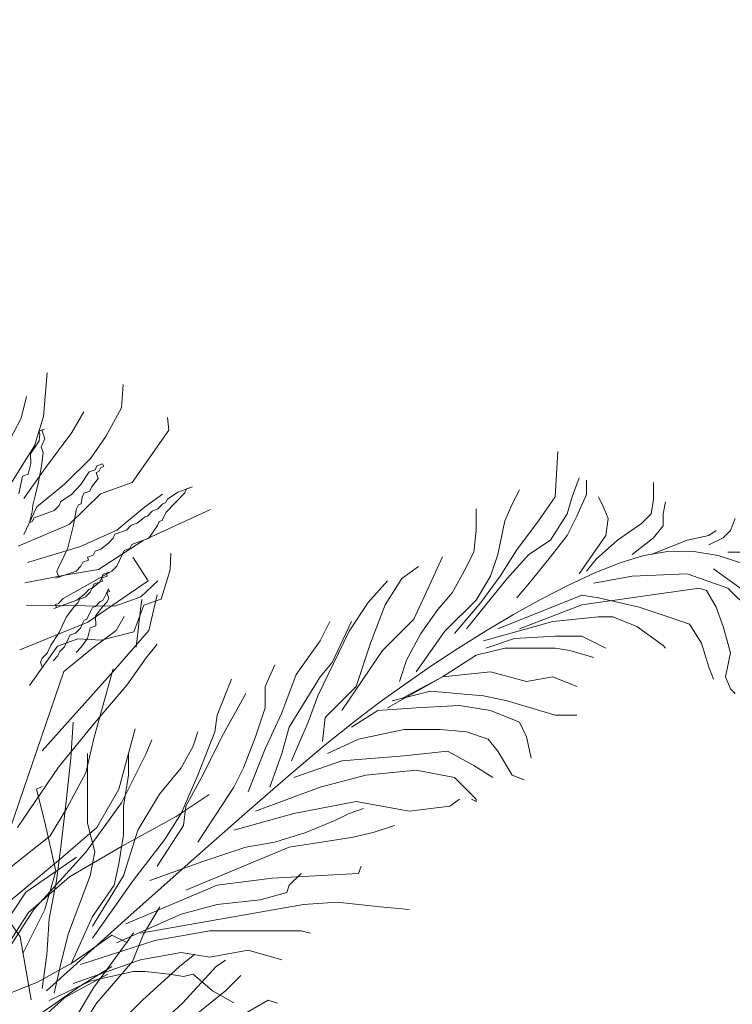
# Model space of a CAD drawing. Units: millimetres. Extents: x 595116 to 630915, y 909473 to 920225.
# Tile 26 of 134: x 629606.562 to 629613.214, y 919171.576 to 919180.767. Entities that reach past the tile are written whole.
import ezdxf

# ---------------------------------------------------------------- set-up
doc = ezdxf.new("R2010")
doc.units = ezdxf.units.MM
doc.layers.add('Dimension', color=3, linetype='Continuous', lineweight=18)
doc.layers.add('L-PLNT', color=85, linetype='Continuous', lineweight=13)
doc.styles.get("Standard").update_dxf_attribs({"font": 'arial.ttf'})
doc.dimstyles.new('ISO-25', dxfattribs={"dimtxt": 9, "dimasz": 6, "dimexe": 1.25, "dimexo": 0.625, "dimtad": 1, "dimlunit": 4, "dimtxsty": 'Standard', "dimcen": 2.5, "dimadec": 0, "dimazin": 0, "dimtfac": 1, "dimtmove": 0, "dimatfit": 3, "dimfxl": 1, "dimarcsym": 0})

# ---------------------------------------------------------------- blocks, each defined once
blk = doc.blocks.new('A$C4FB75ABC')
for p, q in [((2.8876, 3.7608), (2.897, 3.8696)), ((3.0823, 3.7823), (3.0858, 3.8403)), ((2.8322, 3.7571), (2.8454, 3.8105)), ((2.9584, 3.7215), (2.9885, 3.7729)), ((3.043, 3.7114), (3.0823, 3.7823)), ((2.7745, 3.6472), (2.8322, 3.7571)), ((2.8652, 3.6879), (2.8876, 3.7608)), ((3.1994, 3.7272), (3.1962, 3.7584)), ((2.8907, 3.7295), (2.8764, 3.7244)), ((2.8764, 3.7244), (2.8789, 3.7172)), ((2.8835, 3.727), (2.8907, 3.7295)), ((2.8913, 3.7054), (2.8835, 3.727)), ((3.1085, 3.5972), (3.1994, 3.7272)), ((2.8769, 3.7003), (2.856, 3.6684)), ((2.8789, 3.7172), (2.8769, 3.7003)), ((2.8821, 3.6859), (2.8913, 3.7054)), ((2.893, 3.6331), (2.9584, 3.7215)), ((3.0058, 3.6575), (3.043, 3.7114)), ((2.7932, 3.5729), (2.8652, 3.6879)), ((2.8873, 3.6716), (2.8821, 3.6859)), ((4.1608, 3.5609), (4.1668, 3.6742)), ((2.856, 3.6684), (2.8566, 3.6443)), ((2.8833, 3.6377), (2.8873, 3.6716)), ((2.9398, 3.5932), (3.0058, 3.6575)), ((2.8394, 3.5571), (2.893, 3.6331)), ((2.8566, 3.6443), (2.85, 3.6176)), ((2.8746, 3.5941), (2.8833, 3.6377)), ((3.0161, 3.6288), (3.0017, 3.6236)), ((3.0207, 3.6385), (3.0161, 3.6288)), ((3.0187, 3.6216), (3.0258, 3.6242)), ((3.035, 3.6437), (3.0207, 3.6385)), ((3.0258, 3.6242), (3.0304, 3.6339)), ((3.0304, 3.6339), (3.0376, 3.6365)), ((3.0376, 3.6365), (3.035, 3.6437)), ((2.8356, 3.6125), (2.827, 3.5688)), ((2.85, 3.6176), (2.8356, 3.6125)), ((3.0017, 3.6236), (2.9808, 3.5918)), ((3.0075, 3.5852), (3.0238, 3.6072)), ((3.0238, 3.6072), (3.0187, 3.6216)), ((4.2026, 3.5609), (4.2205, 3.6086)), ((4.2384, 3.5668), (4.2384, 3.6026)), ((2.868, 3.5674), (2.8746, 3.5941)), ((2.8712, 3.5361), (2.9398, 3.5932)), ((2.969, 3.5794), (2.9573, 3.5671)), ((2.9808, 3.5918), (2.969, 3.5794)), ((2.9885, 3.5702), (3.0029, 3.5754)), ((3.0029, 3.5754), (3.0075, 3.5852)), ((3.0296, 3.5688), (3.1085, 3.5972)), ((3.2582, 3.5862), (3.2224, 3.5733)), ((3.2393, 3.5713), (3.2439, 3.5811)), ((3.2439, 3.5811), (3.2582, 3.5862)), ((4.0535, 3.543), (4.0714, 3.5788)), ((4.4054, 3.5549), (4.4054, 3.5967)), ((2.8614, 3.5407), (2.868, 3.5674)), ((2.9573, 3.5671), (2.9312, 3.5496)), ((2.9518, 3.4922), (3.0296, 3.5688)), ((2.9819, 3.5435), (2.984, 3.5605)), ((2.984, 3.5605), (2.9885, 3.5702)), ((3.1389, 3.5352), (3.1839, 3.5676)), ((3.1962, 3.5558), (3.1917, 3.5461)), ((3.2224, 3.5733), (3.1962, 3.5558)), ((3.2158, 3.5466), (3.2393, 3.5713)), ((4.1191, 3.5013), (4.1608, 3.5609)), ((4.1907, 3.5192), (4.2026, 3.5609)), ((4.2145, 3.5132), (4.2384, 3.5668)), ((4.2801, 3.537), (4.2682, 3.5609)), ((4.3994, 3.5192), (4.4054, 3.5549)), ((2.8391, 3.4678), (2.8712, 3.5361)), ((2.8594, 3.5238), (2.8614, 3.5407)), ((2.9148, 3.5275), (2.8646, 3.5094)), ((2.9266, 3.5398), (2.9148, 3.5275)), ((2.9312, 3.5496), (2.9266, 3.5398)), ((2.9616, 3.4876), (2.9702, 3.5312)), ((2.9702, 3.5312), (2.9748, 3.541)), ((2.9748, 3.541), (2.9819, 3.5435)), ((3.0703, 3.4781), (3.1389, 3.5352)), ((3.136, 3.4531), (3.303, 3.5294)), ((3.1727, 3.5311), (3.1584, 3.526)), ((3.1845, 3.5435), (3.1727, 3.5311)), ((3.1917, 3.5461), (3.1845, 3.5435)), ((3.1922, 3.522), (3.2158, 3.5466)), ((3.964, 3.4774), (3.964, 3.5311)), ((4.0356, 3.5013), (4.0535, 3.543)), ((4.2921, 3.5072), (4.2801, 3.537)), ((4.4293, 3.5192), (4.4352, 3.549)), ((2.8528, 3.4971), (2.8594, 3.5238)), ((2.8646, 3.5094), (2.86, 3.4997)), ((3.1394, 3.5111), (3.1205, 3.4961)), ((3.1466, 3.5136), (3.1394, 3.5111)), ((3.1584, 3.526), (3.1466, 3.5136)), ((3.1759, 3.4999), (3.1831, 3.5024)), ((3.1831, 3.5024), (3.1922, 3.522)), ((4.1489, 3.4536), (4.1907, 3.5192)), ((4.1907, 3.4655), (4.2145, 3.5132)), ((4.2861, 3.4655), (4.2921, 3.5072)), ((4.3756, 3.4953), (4.3994, 3.5192)), ((4.4293, 3.4893), (4.4293, 3.5192)), ((4.5963, 3.4774), (4.6082, 3.5072)), ((2.8253, 3.4385), (2.9518, 3.4922)), ((2.86, 3.4997), (2.8528, 3.4971)), ((2.9484, 3.4342), (2.9616, 3.4876)), ((2.9797, 3.4374), (3.0703, 3.4781)), ((3.0944, 3.4786), (3.0657, 3.4683)), ((3.1062, 3.491), (3.0944, 3.4786)), ((3.1205, 3.4961), (3.1062, 3.491)), ((3.1503, 3.4583), (3.1713, 3.4901)), ((3.1713, 3.4901), (3.1759, 3.4999)), ((3.958, 3.4238), (3.964, 3.4774)), ((4.0177, 3.4178), (4.0356, 3.5013)), ((4.0654, 3.4297), (4.1191, 3.5013)), ((4.3159, 3.4536), (4.3756, 3.4953)), ((4.4054, 3.4595), (4.4293, 3.4893)), ((4.5426, 3.4655), (4.5605, 3.4774)), ((4.5784, 3.4595), (4.5963, 3.4774)), ((3.0244, 3.3805), (3.136, 3.4531)), ((3.0611, 3.4586), (3.0494, 3.4462)), ((3.0657, 3.4683), (3.0611, 3.4586)), ((3.1073, 3.4428), (3.1503, 3.4583)), ((4.0952, 3.4178), (4.1489, 3.4536)), ((4.1489, 3.4118), (4.1907, 3.4655)), ((4.2205, 3.3701), (4.2861, 3.4655)), ((4.2622, 3.4059), (4.3159, 3.4536)), ((4.3517, 3.4178), (4.4054, 3.4595)), ((4.3994, 3.4178), (4.4889, 3.4536)), ((4.4889, 3.4536), (4.5426, 3.4655)), ((4.5426, 3.4416), (4.5784, 3.4595)), ((2.848, 3.3981), (2.9797, 3.4374)), ((2.9392, 3.4147), (2.9484, 3.4342)), ((3.0304, 3.4313), (3.0161, 3.4262)), ((3.0494, 3.4462), (3.0304, 3.4313)), ((3.0884, 3.4279), (3.1027, 3.433)), ((3.1027, 3.433), (3.1073, 3.4428)), ((4.0237, 3.3641), (4.0654, 3.4297)), ((2.9254, 3.3854), (2.9392, 3.4147)), ((2.9997, 3.4041), (2.9854, 3.3989)), ((3.0115, 3.4164), (2.9972, 3.4112)), ((2.9972, 3.4112), (2.9997, 3.4041)), ((3.0161, 3.4262), (3.0115, 3.4164)), ((3.07, 3.3888), (3.0884, 3.4279)), ((3.1481, 3.3521), (3.1105, 3.4115)), ((3.2028, 3.3799), (3.2043, 3.4209)), ((3.8447, 3.3343), (3.8805, 3.4118)), ((3.9342, 3.3761), (3.958, 3.4238)), ((3.9998, 3.3641), (4.0177, 3.4178)), ((4.0415, 3.3582), (4.0952, 3.4178)), ((4.1012, 3.3522), (4.1489, 3.4118)), ((4.2384, 3.3761), (4.2622, 3.4059)), ((4.322, 3.3969), (4.3813, 3.4152)), ((4.3813, 3.4152), (4.4396, 3.4254)), ((4.4396, 3.4254), (4.5001, 3.426)), ((4.5001, 3.426), (4.5657, 3.4153)), ((4.5657, 3.4153), (4.6395, 3.3917)), ((4.5903, 3.4238), (4.6201, 3.4238)), ((2.9208, 3.3757), (2.9254, 3.3854)), ((2.9403, 3.3665), (3.0244, 3.3805)), ((2.9808, 3.3891), (2.969, 3.3768)), ((2.9854, 3.3989), (2.9808, 3.3891)), ((3.0583, 3.3765), (3.07, 3.3888)), ((3.1805, 3.307), (3.2028, 3.3799)), ((3.7791, 3.3582), (3.8208, 3.388)), ((4.2593, 3.3722), (4.322, 3.3969)), ((4.5545, 3.382), (4.6858, 3.2866)), ((2.8419, 3.3473), (2.9403, 3.3665)), ((2.969, 3.3768), (2.9188, 3.3587)), ((2.9188, 3.3587), (2.926, 3.3613)), ((2.926, 3.3613), (2.9208, 3.3757)), ((2.9369, 3.3085), (3.0583, 3.3765)), ((3.0322, 3.359), (3.0276, 3.3492)), ((3.0367, 3.3687), (3.0322, 3.359)), ((3.0322, 3.359), (3.0465, 3.3642)), ((3.0347, 3.3518), (3.0322, 3.359)), ((3.0511, 3.3739), (3.0367, 3.3687)), ((3.0439, 3.3713), (3.0511, 3.3739)), ((3.0465, 3.3642), (3.0439, 3.3713)), ((3.7373, 3.2926), (3.7791, 3.3582)), ((3.9044, 3.3224), (3.9342, 3.3761)), ((3.964, 3.3045), (3.9998, 3.3641)), ((3.9759, 3.2986), (4.0237, 3.3641)), ((3.9879, 3.2926), (4.0415, 3.3582)), ((4.1935, 3.342), (4.2593, 3.3722)), ((4.2563, 3.3463), (4.3517, 3.3641)), ((4.3517, 3.3641), (4.4889, 3.3701)), ((4.4889, 3.3701), (4.5903, 3.3343)), ((3.0015, 3.3317), (2.9897, 3.3194)), ((2.9986, 3.2497), (3.1481, 3.3521)), ((3.0086, 3.3343), (3.0015, 3.3317)), ((3.004, 3.3246), (3.0086, 3.3343)), ((3.0276, 3.3492), (3.0086, 3.3343)), ((3.0086, 3.3343), (3.0132, 3.3441)), ((3.0132, 3.3441), (3.0347, 3.3518)), ((3.0497, 3.3329), (3.0451, 3.3231)), ((3.0522, 3.3257), (3.0497, 3.3329)), ((3.1297, 3.313), (3.1722, 3.3526)), ((3.6956, 3.2986), (3.7433, 3.3522)), ((3.8089, 3.2568), (3.8447, 3.3343)), ((4.0654, 3.3105), (4.1012, 3.3522)), ((4.1256, 3.3072), (4.1935, 3.342)), ((4.2265, 3.2926), (4.5187, 3.3343)), ((4.5187, 3.3343), (4.5366, 3.3284)), ((4.5903, 3.3343), (4.644, 3.2807)), ((2.9251, 3.2962), (2.9369, 3.3085)), ((2.9897, 3.3194), (2.9708, 3.3045)), ((2.9733, 3.2973), (2.9779, 3.3071)), ((2.9779, 3.3071), (2.9923, 3.3122)), ((2.9923, 3.3122), (3.004, 3.3246)), ((3.0359, 3.3036), (3.0405, 3.3134)), ((3.0405, 3.3134), (3.0451, 3.3231)), ((3.0451, 3.3231), (3.0522, 3.3257)), ((3.0451, 3.3231), (3.0502, 3.3088)), ((3.0502, 3.3088), (3.0456, 3.299)), ((3.0651, 3.2898), (3.1297, 3.313)), ((3.1303, 3.2889), (3.1323, 3.3059)), ((3.1374, 3.2915), (3.1805, 3.307)), ((3.1501, 3.2292), (3.1706, 3.3178)), ((3.8686, 3.2807), (3.9044, 3.3224)), ((4.0177, 3.233), (4.2265, 3.3164)), ((4.0565, 3.2687), (4.1256, 3.3072)), ((4.2265, 3.3164), (4.2682, 3.3105)), ((4.2682, 3.3105), (4.3696, 3.2866)), ((4.5366, 3.3284), (4.5605, 3.2866)), ((2.8457, 3.2919), (3.0651, 3.2898)), ((2.9708, 3.3045), (2.9134, 3.2838)), ((2.9134, 3.2838), (2.9206, 3.2864)), ((2.918, 3.2936), (2.9251, 3.2962)), ((2.9206, 3.2864), (2.918, 3.2936)), ((2.9452, 3.2629), (2.9616, 3.285)), ((2.9616, 3.285), (2.9733, 3.2973)), ((3.0052, 3.2763), (3.0098, 3.2861)), ((3.0098, 3.2861), (3.0169, 3.2887)), ((3.0169, 3.2887), (3.0287, 3.301)), ((3.0339, 3.2867), (3.0175, 3.2646)), ((3.0287, 3.301), (3.0359, 3.3036)), ((3.0456, 3.299), (3.0339, 3.2867)), ((3.1125, 3.2258), (3.1374, 3.2915)), ((3.1182, 3.1873), (3.1303, 3.2889)), ((3.6479, 3.227), (3.6956, 3.2986)), ((3.7015, 3.1972), (3.7373, 3.2926)), ((3.8865, 3.227), (3.964, 3.3045)), ((3.9103, 3.2211), (3.9759, 3.2986)), ((3.9401, 3.233), (3.9879, 3.2926)), ((4.0714, 3.233), (4.2265, 3.2926)), ((4.3696, 3.2866), (4.4412, 3.2628)), ((4.5605, 3.2866), (4.5784, 3.2389)), ((2.936, 3.2434), (2.9452, 3.2629)), ((2.996, 3.2568), (3.0052, 3.2763)), ((3.0175, 3.2646), (3.0181, 3.2405)), ((3.0684, 3.2292), (3.0888, 3.2633)), ((3.8268, 3.2211), (3.8686, 3.2807)), ((3.9871, 3.2274), (4.0565, 3.2687)), ((4.1549, 3.2509), (4.2682, 3.2628)), ((4.2682, 3.2628), (4.304, 3.2628)), ((4.304, 3.2628), (4.3637, 3.2389)), ((4.4412, 3.2628), (4.4949, 3.2449)), ((2.829, 3.1805), (2.9986, 3.2497)), ((2.9269, 3.2238), (2.936, 3.2434)), ((2.9679, 3.2224), (2.9797, 3.2347)), ((2.9797, 3.2347), (2.9842, 3.2445)), ((2.9842, 3.2445), (2.9888, 3.2542)), ((2.9888, 3.2542), (2.996, 3.2568)), ((3.0038, 3.2353), (2.9972, 3.2086)), ((3.0181, 3.2405), (3.0038, 3.2353)), ((3.5763, 3.2032), (3.6001, 3.2509)), ((3.6061, 3.1495), (3.6538, 3.2509)), ((3.7314, 3.1793), (3.8089, 3.2568)), ((3.9819, 3.2032), (4.1549, 3.2509)), ((4.3637, 3.2389), (4.4054, 3.2091)), ((4.4949, 3.2449), (4.5247, 3.1972)), ((4.5784, 3.2389), (4.5963, 3.1734)), ((2.9059, 3.192), (2.9269, 3.2238)), ((2.9229, 3.19), (2.9731, 3.208)), ((2.949, 3.2075), (2.9535, 3.2172)), ((2.9535, 3.2172), (2.9679, 3.2224)), ((2.9731, 3.208), (3.031, 3.2046)), ((2.9972, 3.2086), (2.9808, 3.1865)), ((3.0139, 3.1884), (3.0684, 3.2292)), ((3.031, 3.2046), (3.1125, 3.2258)), ((3.0616, 3.1271), (3.1501, 3.2292)), ((3.5703, 3.066), (3.6479, 3.227)), ((3.791, 3.1555), (3.8268, 3.2211)), ((3.8149, 3.1257), (3.8865, 3.227)), ((3.9185, 3.1843), (3.9871, 3.2274)), ((3.9879, 3.1853), (4.0594, 3.2091)), ((4.0594, 3.2091), (4.1608, 3.2151)), ((4.1608, 3.2151), (4.2265, 3.2151)), ((4.2265, 3.2151), (4.2861, 3.1853)), ((4.4054, 3.2091), (4.4293, 3.1912)), ((2.8529, 3.0918), (2.9229, 3.19)), ((2.8967, 3.1725), (2.9059, 3.192)), ((2.928, 3.1756), (2.9398, 3.188)), ((2.9389, 3.1271), (3.0139, 3.1884)), ((2.9398, 3.188), (2.949, 3.2075)), ((2.9808, 3.1865), (2.969, 3.1742)), ((3.1433, 3.1611), (3.1706, 3.1952)), ((3.5166, 3.1197), (3.5763, 3.2032)), ((3.6658, 3.0899), (3.7015, 3.1972)), ((3.8516, 3.1401), (3.9185, 3.1843)), ((3.964, 3.1674), (4.0356, 3.1853)), ((4.0356, 3.1853), (4.1072, 3.1853)), ((4.1072, 3.1853), (4.1608, 3.1853)), ((4.1608, 3.1853), (4.1966, 3.1793)), ((4.4293, 3.1912), (4.4352, 3.1853)), ((4.5247, 3.1972), (4.5426, 3.1376)), ((2.8804, 3.1504), (2.885, 3.1601)), ((2.885, 3.1601), (2.8967, 3.1725)), ((2.9117, 3.1535), (2.9234, 3.1659)), ((2.9234, 3.1659), (2.928, 3.1756)), ((3.0956, 3.093), (3.1433, 3.1611)), ((3.63, 3.0303), (3.7314, 3.1793)), ((3.8805, 3.1137), (3.964, 3.1674)), ((4.1966, 3.1793), (4.2563, 3.1614)), ((4.5963, 3.1734), (4.5844, 3.1137)), ((2.8856, 3.136), (2.8804, 3.1504)), ((3.4391, 3.0899), (3.4629, 3.1436)), ((3.5763, 3.1137), (3.6061, 3.1495)), ((3.7731, 3.1018), (3.791, 3.1555)), ((3.7873, 3.0958), (3.8516, 3.1401)), ((4.5426, 3.1376), (4.5545, 3.1078)), ((2.7823, 2.6709), (2.9389, 3.1271)), ((2.8844, 2.9296), (3.0616, 3.1271)), ((3.0139, 2.9637), (3.0616, 3.1339)), ((3.4808, 3.0243), (3.5166, 3.1197)), ((3.4987, 2.9885), (3.5763, 3.1137)), ((3.7433, 3.0362), (3.8805, 3.1137)), ((3.7791, 3.0601), (3.8805, 3.1137)), ((3.8805, 3.1137), (3.9998, 3.1257)), ((3.9998, 3.1257), (4.0893, 3.1018)), ((4.0893, 3.1018), (4.1549, 3.1137)), ((4.1549, 3.1137), (4.2145, 3.0899)), ((4.5844, 3.1137), (4.5963, 3.0839)), ((3.0139, 2.9977), (3.0956, 3.093)), ((3.3198, 3.0184), (3.3556, 3.1078)), ((3.4391, 3.0362), (3.4391, 3.0899)), ((3.5882, 3.0124), (3.6658, 3.0899)), ((3.7254, 3.0513), (3.7873, 3.0958)), ((3.3317, 2.9647), (3.3914, 3.072)), ((3.5465, 3.0005), (3.5703, 3.066)), ((3.7552, 3.0541), (3.8507, 3.078)), ((3.8507, 3.078), (3.9819, 3.066)), ((3.9819, 3.066), (4.0415, 3.0541)), ((4.5963, 3.0839), (4.6082, 3.072)), ((3.6611, 3.0024), (3.7254, 3.0513)), ((3.8149, 3.0362), (3.9222, 3.0422)), ((3.9222, 3.0422), (3.9998, 3.0303)), ((4.0415, 3.0541), (4.1608, 3.0184)), ((3.3138, 2.9766), (3.3198, 3.0184)), ((3.4152, 2.9647), (3.4391, 3.0362)), ((3.4391, 2.9349), (3.4808, 3.0243)), ((3.5822, 2.9528), (3.5882, 3.0124)), ((3.6538, 2.9885), (3.7194, 3.0303)), ((3.7194, 3.0303), (3.8149, 3.0362)), ((3.9998, 3.0303), (4.0714, 3.0005)), ((4.1608, 3.0184), (4.2145, 3.0184)), ((2.9253, 2.8888), (3.0139, 2.9977)), ((2.9559, 2.911), (2.9619, 3.0005)), ((3.4808, 2.923), (3.4987, 2.9885)), ((3.5047, 2.9051), (3.5465, 3.0005)), ((3.5886, 2.9442), (3.6611, 3.0024)), ((4.0714, 3.0005), (4.0893, 2.9647)), ((2.9935, 2.8751), (3.0139, 2.9637)), ((3.0752, 2.8343), (3.1161, 2.9841)), ((3.2601, 2.9408), (3.2721, 2.9766)), ((3.2721, 2.8693), (3.3138, 2.9766)), ((3.284, 2.8693), (3.3317, 2.9647)), ((3.3854, 2.8872), (3.4152, 2.9647)), ((3.6717, 2.9587), (3.7851, 2.9826)), ((3.7851, 2.9826), (3.8745, 2.9826)), ((3.8745, 2.9826), (3.9401, 2.9766)), ((3.9401, 2.9766), (3.9938, 2.9587)), ((4.0893, 2.9647), (4.1012, 2.911)), ((3.1433, 2.9228), (3.157, 2.9569)), ((3.2303, 2.8872), (3.2601, 2.9408)), ((3.5019, 2.8714), (3.5886, 2.9442)), ((3.5942, 2.923), (3.6717, 2.9587)), ((3.9938, 2.9587), (4.0177, 2.9289)), ((2.9977, 2.8216), (2.9977, 2.923)), ((3.082, 2.8002), (3.1433, 2.9228)), ((3.0991, 2.8693), (3.0991, 2.923)), ((3.3973, 2.8276), (3.4391, 2.9349)), ((3.451, 2.8395), (3.4808, 2.923)), ((3.63, 2.9051), (3.7851, 2.917)), ((3.7851, 2.917), (3.8924, 2.9289)), ((3.8924, 2.9289), (3.958, 2.8932)), ((4.0177, 2.9289), (4.0535, 2.8693)), ((2.944, 2.8037), (2.9559, 2.911)), ((3.5107, 2.8633), (3.63, 2.9051)), ((3.958, 2.8932), (4.0058, 2.8633)), ((2.8231, 2.739), (2.9253, 2.8888)), ((2.9458, 2.7866), (2.9935, 2.8751)), ((3.0872, 2.7918), (3.0991, 2.8693)), ((3.1766, 2.8216), (3.2303, 2.8872)), ((3.2303, 2.7739), (3.2721, 2.8693)), ((3.2422, 2.7918), (3.284, 2.8693)), ((3.3615, 2.8395), (3.3854, 2.8872)), ((3.3951, 2.779), (3.5019, 2.8714)), ((3.5763, 2.8395), (3.6896, 2.8693)), ((3.6896, 2.8693), (3.8149, 2.8812)), ((3.8149, 2.8812), (3.9103, 2.8633)), ((4.0535, 2.8693), (4.0833, 2.8574)), ((2.8708, 2.8343), (2.8844, 2.8411)), ((3.9103, 2.8633), (3.964, 2.8097)), ((2.8913, 2.7526), (2.8708, 2.8343)), ((2.9977, 2.7501), (2.9977, 2.8216)), ((3.0207, 2.739), (3.0752, 2.8343)), ((3.1229, 2.7322), (3.1766, 2.8216)), ((3.2183, 2.7662), (3.3, 2.8207)), ((3.2721, 2.7024), (3.3615, 2.8395)), ((3.4152, 2.7799), (3.5763, 2.8395)), ((2.9321, 2.6964), (2.944, 2.8037)), ((2.9935, 2.6777), (3.082, 2.8002)), ((3.0872, 2.7203), (3.0872, 2.7918)), ((3.2363, 2.7441), (3.2422, 2.7918)), ((3.5107, 2.7739), (3.6658, 2.8037)), ((3.6658, 2.8037), (3.797, 2.7799)), ((3.797, 2.7799), (3.8984, 2.7918)), ((3.8984, 2.7918), (3.9222, 2.8097)), ((3.964, 2.8037), (3.9521, 2.8097)), ((3.964, 2.8097), (3.964, 2.8037)), ((2.9049, 2.7185), (2.9458, 2.7866)), ((3.1886, 2.7083), (3.2303, 2.7739)), ((3.2623, 2.6619), (3.3951, 2.779)), ((3.3615, 2.7322), (3.5107, 2.7739)), ((3.6121, 2.756), (3.6479, 2.7739)), ((3.6479, 2.7739), (3.6837, 2.7858)), ((2.9185, 2.63), (2.8913, 2.7526)), ((3.0156, 2.6785), (2.9977, 2.7501)), ((3.082, 2.6913), (3.2183, 2.7662)), ((3.1707, 2.6428), (3.2363, 2.7441)), ((3.5405, 2.7262), (3.6121, 2.756)), ((3.7075, 2.7262), (3.7612, 2.7441)), ((2.7414, 2.5891), (2.9049, 2.7185)), ((2.9253, 2.6572), (3.0207, 2.739)), ((3.0752, 2.6487), (3.0872, 2.7203)), ((3.0872, 2.6189), (3.1229, 2.7322)), ((3.4629, 2.7024), (3.5405, 2.7262)), ((3.6538, 2.7143), (3.7075, 2.7262)), ((2.9201, 2.607), (2.9321, 2.6964)), ((3.111, 2.607), (3.1886, 2.7083)), ((3.3914, 2.6904), (3.4629, 2.7024)), ((3.4987, 2.6904), (3.6538, 2.7143)), ((2.864, 2.5347), (2.9935, 2.6777)), ((2.9526, 2.6164), (3.082, 2.6913)), ((3.0036, 2.6189), (3.0156, 2.6785)), ((3.2422, 2.5831), (3.4987, 2.6904)), ((3.284, 2.6547), (3.3914, 2.6904)), ((2.7209, 2.487), (2.9253, 2.6572)), ((2.8442, 2.5778), (2.9704, 2.6651)), ((3.0633, 2.5951), (3.0752, 2.6487)), ((3.0976, 2.5149), (3.2623, 2.6619)), ((3.1528, 2.607), (3.284, 2.6547)), ((2.8913, 2.5347), (2.9185, 2.63)), ((3.457, 2.6129), (3.6717, 2.6249)), ((3.4987, 2.5951), (3.5286, 2.6249)), ((3.6717, 2.6249), (3.6777, 2.6428)), ((2.8504, 2.5279), (2.9526, 2.6164)), ((2.9022, 2.5116), (2.9201, 2.607)), ((2.95, 2.4758), (3.0036, 2.6189)), ((3.0096, 2.4937), (3.0872, 2.6189)), ((3.0096, 2.4639), (3.111, 2.607)), ((3.3198, 2.5951), (3.457, 2.6129)), ((2.786, 2.4905), (2.8442, 2.5778)), ((3.0096, 2.5176), (3.0633, 2.5951)), ((3.0931, 2.4997), (3.3198, 2.5951)), ((3.4272, 2.5593), (3.4928, 2.5772)), ((3.4928, 2.5772), (3.4987, 2.5951)), ((2.8299, 2.4666), (2.7686, 2.5551)), ((3.1289, 2.4758), (3.5345, 2.5474)), ((3.2303, 2.5235), (3.3198, 2.5474)), ((3.3198, 2.5474), (3.4272, 2.5593)), ((3.5345, 2.5474), (3.618, 2.5533)), ((3.618, 2.5533), (3.7254, 2.5414)), ((2.7891, 2.4325), (2.8504, 2.5279)), ((2.8027, 2.4393), (2.864, 2.5347)), ((2.8368, 2.4257), (2.8913, 2.5347)), ((3.0693, 2.452), (3.2303, 2.5235)), ((3.1365, 2.4734), (3.1774, 2.5415)), ((3.7254, 2.5414), (3.797, 2.5354)), ((2.895, 2.333), (3.0976, 2.5149)), ((2.8963, 2.4222), (2.9022, 2.5116)), ((2.9559, 2.3983), (3.0096, 2.5176)), ((2.9321, 2.4043), (2.95, 2.4758)), ((3.0962, 2.4544), (3.1115, 2.4773)), ((3.1093, 2.4053), (3.1365, 2.4734)), ((3.1647, 2.4579), (3.3019, 2.4818)), ((3.3019, 2.4818), (3.4152, 2.4818)), ((3.4152, 2.4818), (3.5286, 2.4818)), ((3.5286, 2.4818), (3.5524, 2.4758)), ((2.8572, 2.31), (2.8299, 2.4666)), ((2.9607, 2.4032), (3.0578, 2.4711)), ((2.9798, 2.3983), (3.1647, 2.4579)), ((3.0123, 2.3401), (3.0962, 2.4544)), ((3.0578, 2.4711), (3.0966, 2.4517)), ((3.1289, 2.4102), (3.2303, 2.4281)), ((3.2303, 2.4281), (3.3019, 2.4162)), ((3.3019, 2.4162), (3.3973, 2.4341)), ((3.3973, 2.4341), (3.4808, 2.4102)), ((2.8733, 2.3546), (2.9607, 2.4032)), ((2.8844, 2.3387), (2.8963, 2.4222)), ((2.9142, 2.3268), (2.9321, 2.4043)), ((2.9619, 2.3506), (3.1289, 2.4102)), ((3.0207, 2.3031), (3.1093, 2.4053)), ((3.2259, 2.3934), (3.264, 2.4239)), ((3.3174, 2.3934), (3.3403, 2.4087)), ((2.9801, 2.3449), (3.0578, 2.3935)), ((3.0036, 2.3566), (3.111, 2.3804)), ((3.111, 2.3804), (3.1408, 2.3804)), ((3.1344, 2.3096), (3.2259, 2.3934)), ((3.1408, 2.3804), (3.2005, 2.3745)), ((3.2335, 2.302), (3.3174, 2.3934)), ((2.7277, 2.2964), (2.8733, 2.3546)), ((2.9022, 2.3089), (3.0036, 2.3566)), ((2.9413, 2.3158), (3.0481, 2.3741)), ((3.2005, 2.3745), (3.2363, 2.3685)), ((3.2363, 2.3685), (3.2601, 2.3745)), ((3.2601, 2.3745), (3.3079, 2.3327)), ((3.3403, 2.3324), (3.3784, 2.3706)), ((2.8539, 2.2576), (2.9801, 2.3449)), ((2.9666, 2.2638), (3.0123, 2.3401)), ((3.264, 2.2715), (3.3403, 2.3324)), ((3.3079, 2.3327), (3.3615, 2.3029)), ((2.8539, 2.2382), (2.9413, 2.3158)), ((2.9321, 2.167), (3.0207, 2.3031)), ((3.0505, 2.2257), (3.1344, 2.3096)), ((3.142, 2.2181), (3.2335, 2.302)), ((3.3937, 2.2791), (3.447, 2.3096)), ((3.447, 2.3096), (3.4699, 2.302))]:
    blk.add_line(p, q)
blk = doc.blocks.new('*D216')
at = {"layer": 'Defpoints', "color": 0, "transparency": 16777216}
for p in [(629743.5408, 919411.9276), (629505.0408, 919411.8279), (629743.5408, 918832.3776)]:
    blk.add_point(p, dxfattribs=at)
at = {"layer": 'Dimension', "color": 0, "lineweight": -2, "transparency": 16777216}
for p, q in [((629743.5408, 919411.3026), (629743.5408, 918831.1276)), ((629505.0408, 919411.2029), (629505.0408, 918831.1276)), ((629511.0408, 918832.3776), (629737.5408, 918832.3776))]:
    blk.add_line(p, q, dxfattribs=at)
at = {"layer": 'Dimension', "color": 0, "transparency": 16777216}
for points in [[(629511.0408, 918833.3776), (629511.0408, 918831.3776), (629505.0408, 918832.3776)], [(629737.5408, 918833.3776), (629737.5408, 918831.3776), (629743.5408, 918832.3776)]]:
    blk.add_solid(points, dxfattribs=at)
at = {"layer": 'Dimension', "color": 0, "transparency": 16777216, "insert": (629624.2908, 918837.656), "char_height": 9, "attachment_point": 5}
blk.add_mtext('19\'-10 1/2"', dxfattribs=at)

msp = doc.modelspace()

# ---------------------------------------------------------------- block references
at = {"layer": 'L-PLNT', "xscale": 3.753413438031968, "yscale": 3.753413438031968, "zscale": 3.753413438031968}
msp.add_blockref('A$C4FB75ABC', (629595.9442, 919162.9458), dxfattribs=at)

# ---------------------------------------------------------------- dimensions: what is measured, and where the dimension line sits
at = {"layer": 'Dimension'}
dim = msp.add_linear_dim(base=(629743.5408, 918832.3776), p1=(629505.0408, 919411.8279), p2=(629743.5408, 919411.9276), dimstyle='ISO-25', override={"dimdec": 1, "dimlfac": 1, "dimrnd": 0, "dimzin": 1, "dimdsep": 46, "dimlunit": 4, "dimfrac": 2}, dxfattribs=at)
dim.commit()
dim.dimension.update_dxf_attribs({"geometry": '*D216', "text_midpoint": (629624.2908, 918837.656)})

doc.saveas('drawing.dxf')
